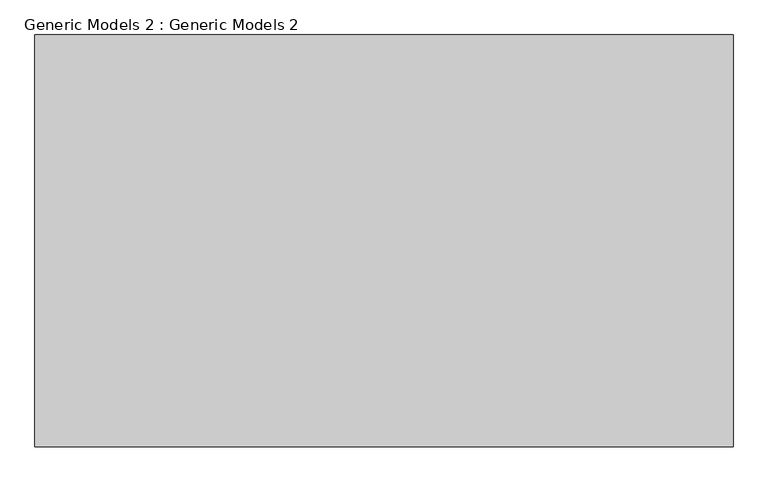
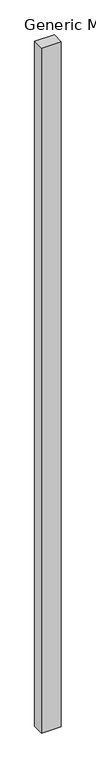
"""IFC4 building model written with IfcOpenShell, lengths in millimetres: proxy geometry, Generic Models 2 : Generic Models 2."""

from ifc_helpers import new_model, si_unit, frame, origin, place, context, project, spatial, polyline, outline, extrude, source, transform, mapped, element, save


def generic_models_2_generic_models_2_5afbfd34(model_context):
    return source(origin(), model_context, "Body", "SweptSolid", [
        extrude(outline(polyline([(5043.9964352, -14078.0808221), (5043.9964352, -14858.1778294), (3720.7908965, -14858.1778294), (3720.7908965, -14078.0808221), (5043.9964352, -14078.0808221)])), frame((0.0, 0.0, 6579.2511164), z_axis=(0.0, 0.0, 1.0), x_axis=(1.0, 0.0, 0.0)), (0.0, 0.0, 1.0), 48894.3488836),
    ])


if __name__ == "__main__":
    model = new_model("IFC4")
    model_context = context("Model", 3, world=origin())
    ifc_project = project(units=[si_unit("LENGTHUNIT", "METRE", prefix="MILLI")], contexts=[model_context])
    site = spatial("IfcSite", under=ifc_project)
    building = spatial("IfcBuilding", under=site)
    placement = place(None, origin())
    generic_models_2_generic_models_2_shape = generic_models_2_generic_models_2_5afbfd34(model_context)
    element("IfcBuildingElementProxy", 1, Name="Generic Models 2 : Generic Models 2", ObjectType="Generic Models 2 : Generic Models 2", at=placement, inside=building, context=model_context, shape_type="MappedRepresentation", body=[
        mapped(generic_models_2_generic_models_2_shape, transform((0.0, 0.0, 0.0), x_axis=(1.0, 0.0, 0.0), y_axis=(0.0, 1.0, 0.0), z_axis=(0.0, 0.0, 1.0))),
    ])
    save(model, "model.ifc")
